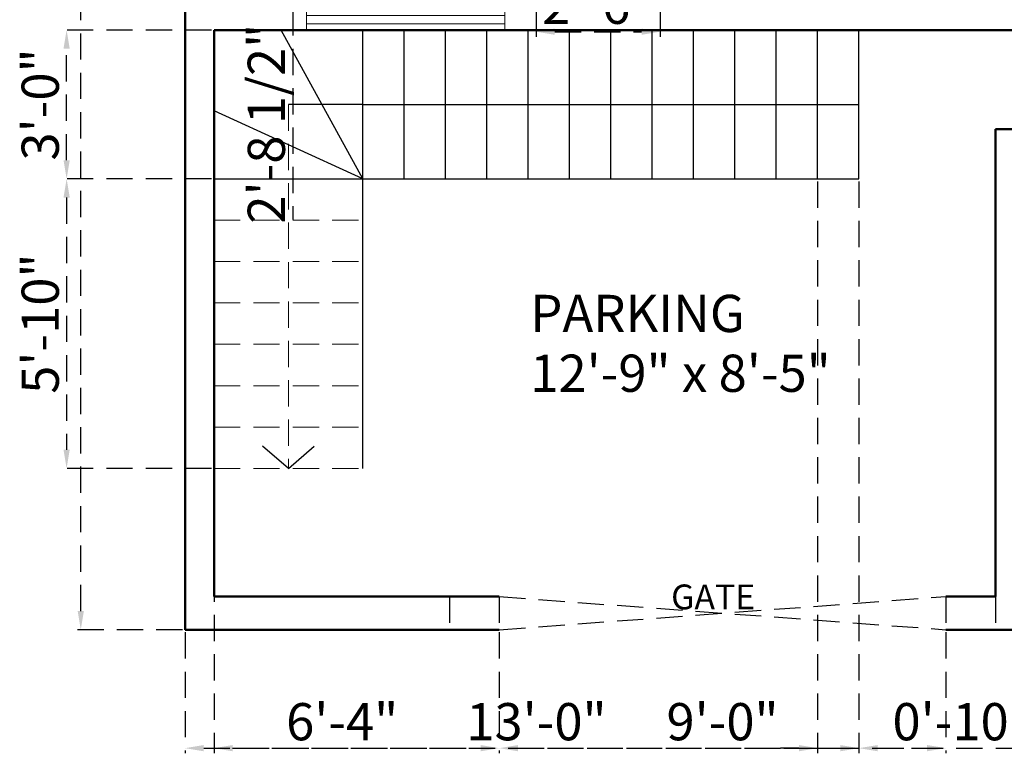
# Model space of a CAD drawing. Units: inches. Extents: x 3209 to 7144, y 1281 to 3076.
# Tile 1 of 5: x 3236 to 3474, y 1281 to 1459. Entities that reach past the tile are written whole.
import ezdxf

# ---------------------------------------------------------------- set-up
doc = ezdxf.new("R2010")
doc.units = ezdxf.units.IN
doc.linetypes.add('HIDDEN', pattern=[9.525, 6.35, -3.175])
for name, color, linetype, lineweight in [('A-ANNO-DIMS', 244, 'HIDDEN', 18), ('A-ANNO-TEXT', 7, 'Continuous', 18), ('A-AREA-IDEN', 7, 'Continuous', 25), ('A-DOOR-GATE', 244, 'HIDDEN', 25), ('A-FLOR-STRS', 7, 'Continuous', 25), ('A-FLOR-STRS-HIDN', 7, 'HIDDEN', 18), ('A-GLAZ', 4, 'Continuous', 18), ('A-WALL', 7, 'Continuous', 50)]:
    doc.layers.add(name, color=color, linetype=linetype, lineweight=lineweight)
doc.styles.get("Standard").update_dxf_attribs({"font": 'arial.ttf'})
doc.dimstyles.new('ISO-25', dxfattribs={"dimtxt": 9, "dimasz": 4.5, "dimexe": 1.25, "dimexo": 0.625, "dimtad": 1, "dimdec": 0, "dimlunit": 3, "dimtxsty": 'Standard', "dimcen": 2.5, "dimadec": 0, "dimazin": 0, "dimtfac": 1, "dimtdec": 0, "dimtmove": 0, "dimatfit": 3, "dimfxl": 1, "dimarcsym": 0})

# ---------------------------------------------------------------- blocks, each defined once
blk = doc.blocks.new('*D15')
at = {"layer": 'A-ANNO-DIMS', "color": 0, "lineweight": -2, "transparency": 16777216}
for p, q in [((3275.31, 1851.27), (3249.46, 1851.27)), ((3250.71, 1315.77), (3250.71, 1846.77)), ((3275.31, 1311.27), (3249.46, 1311.27))]:
    blk.add_line(p, q, dxfattribs=at)
at = {"layer": 'A-ANNO-DIMS', "color": 0, "transparency": 16777216}
for points in [[(3249.96, 1846.77), (3251.46, 1846.77), (3250.71, 1851.27)], [(3249.96, 1315.77), (3251.46, 1315.77), (3250.71, 1311.27)]]:
    blk.add_solid(points, dxfattribs=at)
at = {"layer": 'Defpoints', "color": 0, "transparency": 16777216}
for p in [(3250.71, 1851.27), (3275.94, 1851.27), (3275.94, 1311.27)]:
    blk.add_point(p, dxfattribs=at)
at = {"layer": 'A-ANNO-DIMS', "color": 0, "transparency": 16777216, "insert": (3245.51, 1581.27), "char_height": 9, "attachment_point": 5, "rotation": 90}
blk.add_mtext("45'", dxfattribs=at)
blk = doc.blocks.new('WINDOW-48IN-WALL5')
for p, q in [((0, 5), (0, 0)), ((48, 5), (48, 0)), ((0, 3.5), (48, 3.5)), ((0, 1.5), (48, 1.5))]:
    blk.add_line(p, q)
blk = doc.blocks.new('*D57')
at = {"layer": 'A-ANNO-DIMS', "color": 0, "lineweight": -2, "transparency": 16777216}
for p, q in [((3360.88, 1460.64), (3360.88, 1454.62)), ((3390.88, 1460.64), (3390.88, 1454.62)), ((3365.38, 1455.87), (3386.38, 1455.87))]:
    blk.add_line(p, q, dxfattribs=at)
at = {"layer": 'A-ANNO-DIMS', "color": 0, "transparency": 16777216}
for points in [[(3365.38, 1456.62), (3365.38, 1455.12), (3360.88, 1455.87)], [(3386.38, 1456.62), (3386.38, 1455.12), (3390.88, 1455.87)]]:
    blk.add_solid(points, dxfattribs=at)
at = {"layer": 'Defpoints', "color": 0, "transparency": 16777216}
for p in [(3360.88, 1461.27), (3390.88, 1461.27), (3390.88, 1455.87)]:
    blk.add_point(p, dxfattribs=at)
at = {"layer": 'A-ANNO-DIMS', "color": 0, "transparency": 16777216, "insert": (3375.88, 1461.09), "char_height": 9, "attachment_point": 5}
blk.add_mtext('2\'-6"', dxfattribs=at)
blk = doc.blocks.new('*D63')
at = {"layer": 'A-ANNO-DIMS', "color": 0, "lineweight": -2, "transparency": 16777216}
for p, q in [((3307.07, 1493.93), (3300.79, 1493.93)), ((3302.04, 1489.43), (3302.04, 1465.77)), ((3307.07, 1461.27), (3300.79, 1461.27)), ((3302.04, 1461.27), (3302.04, 1410.47))]:
    blk.add_line(p, q, dxfattribs=at)
at = {"layer": 'A-ANNO-DIMS', "color": 0, "transparency": 16777216}
for points in [[(3301.29, 1489.43), (3302.79, 1489.43), (3302.04, 1493.93)], [(3301.29, 1465.77), (3302.79, 1465.77), (3302.04, 1461.27)]]:
    blk.add_solid(points, dxfattribs=at)
at = {"layer": 'Defpoints', "color": 0, "transparency": 16777216}
for p in [(3307.69, 1493.93), (3302.04, 1461.27), (3307.69, 1461.27)]:
    blk.add_point(p, dxfattribs=at)
at = {"layer": 'A-ANNO-DIMS', "color": 0, "transparency": 16777216, "insert": (3296.76, 1433.62), "char_height": 9, "attachment_point": 5, "rotation": 90}
blk.add_mtext('2\'-8 1/2"', dxfattribs=at)
blk = doc.blocks.new('*D64')
at = {"layer": 'A-ANNO-DIMS', "color": 0, "lineweight": -2, "transparency": 16777216}
for p, q in [((3351.94, 1310.64), (3351.94, 1281.37)), ((3459.94, 1310.64), (3459.94, 1281.37)), ((3356.44, 1282.62), (3455.44, 1282.62))]:
    blk.add_line(p, q, dxfattribs=at)
at = {"layer": 'A-ANNO-DIMS', "color": 0, "transparency": 16777216}
for points in [[(3356.44, 1283.37), (3356.44, 1281.87), (3351.94, 1282.62)], [(3455.44, 1283.37), (3455.44, 1281.87), (3459.94, 1282.62)]]:
    blk.add_solid(points, dxfattribs=at)
at = {"layer": 'Defpoints', "color": 0, "transparency": 16777216}
for p in [(3351.94, 1311.27), (3459.94, 1311.27), (3459.94, 1282.62)]:
    blk.add_point(p, dxfattribs=at)
at = {"layer": 'A-ANNO-DIMS', "color": 0, "transparency": 16777216, "insert": (3405.94, 1287.85), "char_height": 9, "attachment_point": 5}
blk.add_mtext('9\'-0"', dxfattribs=at)
blk = doc.blocks.new('*D65')
at = {"layer": 'A-ANNO-DIMS', "color": 0, "lineweight": -2, "transparency": 16777216}
for p, q in [((3275.94, 1310.64), (3275.94, 1281.37)), ((3351.94, 1310.64), (3351.94, 1281.37)), ((3280.44, 1282.62), (3347.44, 1282.62))]:
    blk.add_line(p, q, dxfattribs=at)
at = {"layer": 'A-ANNO-DIMS', "color": 0, "transparency": 16777216}
for points in [[(3280.44, 1283.37), (3280.44, 1281.87), (3275.94, 1282.62)], [(3347.44, 1283.37), (3347.44, 1281.87), (3351.94, 1282.62)]]:
    blk.add_solid(points, dxfattribs=at)
at = {"layer": 'Defpoints', "color": 0, "transparency": 16777216}
for p in [(3275.94, 1311.27), (3351.94, 1311.27), (3351.94, 1282.62)]:
    blk.add_point(p, dxfattribs=at)
at = {"layer": 'A-ANNO-DIMS', "color": 0, "transparency": 16777216, "insert": (3313.94, 1287.85), "char_height": 9, "attachment_point": 5}
blk.add_mtext('6\'-4"', dxfattribs=at)
blk = doc.blocks.new('*D69')
at = {"layer": 'A-ANNO-DIMS', "color": 0, "lineweight": -2, "transparency": 16777216}
for p, q in [((3282.31, 1456.27), (3246.04, 1456.27)), ((3247.29, 1424.77), (3247.29, 1451.77)), ((3282.31, 1420.27), (3246.04, 1420.27))]:
    blk.add_line(p, q, dxfattribs=at)
at = {"layer": 'A-ANNO-DIMS', "color": 0, "transparency": 16777216}
for points in [[(3246.54, 1451.77), (3248.04, 1451.77), (3247.29, 1456.27)], [(3246.54, 1424.77), (3248.04, 1424.77), (3247.29, 1420.27)]]:
    blk.add_solid(points, dxfattribs=at)
at = {"layer": 'Defpoints', "color": 0, "transparency": 16777216}
for p in [(3247.29, 1456.27), (3282.94, 1456.27), (3282.94, 1420.27)]:
    blk.add_point(p, dxfattribs=at)
at = {"layer": 'A-ANNO-DIMS', "color": 0, "transparency": 16777216, "insert": (3242.07, 1438.27), "char_height": 9, "attachment_point": 5, "rotation": 90}
blk.add_mtext('3\'-0"', dxfattribs=at)
blk = doc.blocks.new('*D70')
at = {"layer": 'A-ANNO-DIMS', "color": 0, "lineweight": -2, "transparency": 16777216}
for p, q in [((3282.31, 1420.27), (3246.04, 1420.27)), ((3247.29, 1415.77), (3247.29, 1354.77)), ((3282.31, 1350.27), (3246.04, 1350.27))]:
    blk.add_line(p, q, dxfattribs=at)
at = {"layer": 'A-ANNO-DIMS', "color": 0, "transparency": 16777216}
for points in [[(3246.54, 1415.77), (3248.04, 1415.77), (3247.29, 1420.27)], [(3246.54, 1354.77), (3248.04, 1354.77), (3247.29, 1350.27)]]:
    blk.add_solid(points, dxfattribs=at)
at = {"layer": 'Defpoints', "color": 0, "transparency": 16777216}
for p in [(3282.94, 1420.27), (3247.29, 1350.27), (3282.94, 1350.27)]:
    blk.add_point(p, dxfattribs=at)
at = {"layer": 'A-ANNO-DIMS', "color": 0, "transparency": 16777216, "insert": (3242.07, 1385.27), "char_height": 9, "attachment_point": 5, "rotation": 90}
blk.add_mtext('5\'-10"', dxfattribs=at)
blk = doc.blocks.new('*D71')
at = {"layer": 'A-ANNO-DIMS', "color": 0, "lineweight": -2, "transparency": 16777216}
for p, q in [((3282.94, 1419.64), (3282.94, 1281.37)), ((3438.94, 1419.64), (3438.94, 1281.37)), ((3287.44, 1282.62), (3434.44, 1282.62))]:
    blk.add_line(p, q, dxfattribs=at)
at = {"layer": 'A-ANNO-DIMS', "color": 0, "transparency": 16777216}
for points in [[(3287.44, 1283.37), (3287.44, 1281.87), (3282.94, 1282.62)], [(3434.44, 1283.37), (3434.44, 1281.87), (3438.94, 1282.62)]]:
    blk.add_solid(points, dxfattribs=at)
at = {"layer": 'Defpoints', "color": 0, "transparency": 16777216}
for p in [(3282.94, 1420.27), (3438.94, 1420.27), (3438.94, 1282.62)]:
    blk.add_point(p, dxfattribs=at)
at = {"layer": 'A-ANNO-DIMS', "color": 0, "transparency": 16777216, "insert": (3360.94, 1287.85), "char_height": 9, "attachment_point": 5}
blk.add_mtext('13\'-0"', dxfattribs=at)
blk = doc.blocks.new('*D72')
at = {"layer": 'A-ANNO-DIMS', "color": 0, "lineweight": -2, "transparency": 16777216}
for p, q in [((3428.94, 1419.64), (3428.94, 1281.37)), ((3438.94, 1419.64), (3438.94, 1281.37)), ((3424.44, 1282.62), (3419.94, 1282.62)), ((3428.94, 1282.62), (3438.94, 1282.62)), ((3443.44, 1282.62), (3480.11, 1282.62))]:
    blk.add_line(p, q, dxfattribs=at)
at = {"layer": 'A-ANNO-DIMS', "color": 0, "transparency": 16777216}
for points in [[(3424.44, 1283.37), (3424.44, 1281.87), (3428.94, 1282.62)], [(3443.44, 1283.37), (3443.44, 1281.87), (3438.94, 1282.62)]]:
    blk.add_solid(points, dxfattribs=at)
at = {"layer": 'Defpoints', "color": 0, "transparency": 16777216}
for p in [(3428.94, 1420.27), (3438.94, 1420.27), (3438.94, 1282.62)]:
    blk.add_point(p, dxfattribs=at)
at = {"layer": 'A-ANNO-DIMS', "color": 0, "transparency": 16777216, "insert": (3464.02, 1287.85), "char_height": 9, "attachment_point": 5}
blk.add_mtext('0\'-10"', dxfattribs=at)

msp = doc.modelspace()

# ---------------------------------------------------------------- linework, layer by layer
at = {"layer": 'A-DOOR-GATE'}
for p, q in [((3339.94, 1319.27), (3339.94, 1311.27)), ((3351.94, 1319.27), (3351.94, 1311.27)), ((3351.94, 1319.27), (3459.94, 1311.27)), ((3351.94, 1311.27), (3459.94, 1319.27)), ((3459.94, 1319.27), (3459.94, 1311.27)), ((3471.94, 1319.27), (3471.94, 1311.27))]:
    msp.add_line(p, q, dxfattribs=at)
at = {"layer": 'A-FLOR-STRS'}
for p, q in [((3318.94, 1420.27), (3299.18, 1456.27)), ((3318.94, 1350.27), (3318.94, 1456.27)), ((3318.94, 1420.27), (3318.94, 1456.27)), ((3328.94, 1420.27), (3328.94, 1456.27)), ((3338.94, 1420.27), (3338.94, 1456.27)), ((3348.94, 1420.27), (3348.94, 1456.27)), ((3358.94, 1420.27), (3358.94, 1456.27)), ((3368.94, 1420.27), (3368.94, 1456.27)), ((3378.94, 1420.27), (3378.94, 1456.27)), ((3388.94, 1420.27), (3388.94, 1456.27)), ((3398.94, 1420.27), (3398.94, 1456.27)), ((3408.94, 1420.27), (3408.94, 1456.27)), ((3418.94, 1420.27), (3418.94, 1456.27)), ((3428.94, 1420.27), (3428.94, 1456.27)), ((3438.94, 1420.27), (3438.94, 1456.27)), ((3318.94, 1420.27), (3282.94, 1436.76)), ((3318.94, 1438.27), (3300.94, 1438.27)), ((3318.94, 1438.27), (3438.94, 1438.27)), ((3282.94, 1420.27), (3438.94, 1420.27)), ((3282.94, 1420.27), (3318.94, 1420.27)), ((3300.94, 1350.27), (3294.69, 1355.67)), ((3300.94, 1350.27), (3307.18, 1355.67))]:
    msp.add_line(p, q, dxfattribs=at)
at = {"layer": 'A-FLOR-STRS-HIDN'}
for p, q in [((3300.94, 1438.27), (3300.94, 1350.27)), ((3282.94, 1410.27), (3318.94, 1410.27)), ((3282.94, 1400.27), (3318.94, 1400.27)), ((3282.94, 1390.27), (3318.94, 1390.27)), ((3282.94, 1380.27), (3318.94, 1380.27)), ((3282.94, 1370.27), (3318.94, 1370.27)), ((3282.94, 1360.27), (3318.94, 1360.27)), ((3282.94, 1350.27), (3318.94, 1350.27))]:
    msp.add_line(p, q, dxfattribs=at)
at = {"layer": 'A-WALL'}
for p, q in [((3275.94, 1311.27), (3275.94, 1851.27)), ((3282.94, 1319.27), (3282.94, 1456.27)), ((3282.94, 1456.27), (3476.94, 1456.27)), ((3471.94, 1432.27), (3471.94, 1319.27)), ((3482.94, 1432.27), (3471.94, 1432.27)), ((3351.94, 1319.27), (3282.94, 1319.27)), ((3471.94, 1319.27), (3459.94, 1319.27)), ((3351.94, 1311.27), (3275.94, 1311.27)), ((3635.94, 1311.27), (3459.94, 1311.27))]:
    msp.add_line(p, q, dxfattribs=at)

# ---------------------------------------------------------------- block references
at = {"layer": 'A-GLAZ'}
msp.add_blockref('WINDOW-48IN-WALL5', (3305.28, 1456.27), dxfattribs=at)

# ---------------------------------------------------------------- texts
at = {"layer": 'A-ANNO-TEXT'}
msp.add_text('GATE', height=6, dxfattribs=at).set_placement((3393.51, 1316.19))
at = {"layer": 'A-AREA-IDEN'}
for s, p in [('PARKING', (3359.45, 1383.24)), ('12\'-9" x 8\'-5"', (3359.45, 1368.78))]:
    msp.add_text(s, height=9, dxfattribs=at).set_placement(p)

# ---------------------------------------------------------------- dimensions: what is measured, and where the dimension line sits
at = {"layer": 'A-ANNO-DIMS'}
for base, p1, p2, angle, override, picture, middle in [((3250.71, 1851.27), (3275.94, 1311.27), (3275.94, 1851.27), 90, {"dimclrd": 0, "dimclre": 0, "dimclrt": 0}, '*D15', (3245.51, 1581.27)), ((3302.04, 1461.27), (3307.69, 1493.93), (3307.69, 1461.27), 270, {"dimdec": 1, "dimlfac": 1, "dimrnd": 0, "dimzin": 1, "dimdsep": 46, "dimlunit": 4, "dimfrac": 2}, '*D63', (3296.76, 1433.62)), ((3247.29, 1456.27), (3282.94, 1420.27), (3282.94, 1456.27), 90, {"dimdec": 1, "dimlfac": 1, "dimrnd": 0, "dimzin": 1, "dimdsep": 46, "dimlunit": 4, "dimfrac": 2}, '*D69', (3242.07, 1438.27)), ((3247.29, 1350.27), (3282.94, 1420.27), (3282.94, 1350.27), 90, {"dimdec": 1, "dimlfac": 1, "dimrnd": 0, "dimzin": 1, "dimdsep": 46, "dimlunit": 4, "dimfrac": 2}, '*D70', (3242.07, 1385.27))]:
    dim = msp.add_linear_dim(base=base, p1=p1, p2=p2, angle=angle, dimstyle='ISO-25', override=override, dxfattribs=at)
    dim.commit()
    dim.dimension.update_dxf_attribs({"geometry": picture, "text_midpoint": middle})
for base, p1, p2, picture, middle in [((3390.88, 1455.87), (3360.88, 1461.27), (3390.88, 1461.27), '*D57', (3375.88, 1461.09)), ((3438.94, 1282.62), (3282.94, 1420.27), (3438.94, 1420.27), '*D71', (3360.94, 1287.85)), ((3438.94, 1282.62), (3428.94, 1420.27), (3438.94, 1420.27), '*D72', (3464.02, 1287.85)), ((3351.94, 1282.62), (3275.94, 1311.27), (3351.94, 1311.27), '*D65', (3313.94, 1287.85)), ((3459.94, 1282.62), (3351.94, 1311.27), (3459.94, 1311.27), '*D64', (3405.94, 1287.85))]:
    dim = msp.add_linear_dim(base=base, p1=p1, p2=p2, dimstyle='ISO-25', override={"dimdec": 1, "dimlfac": 1, "dimrnd": 0, "dimzin": 1, "dimdsep": 46, "dimlunit": 4, "dimfrac": 2}, dxfattribs=at)
    dim.commit()
    dim.dimension.update_dxf_attribs({"geometry": picture, "text_midpoint": middle})

doc.saveas('drawing.dxf')
